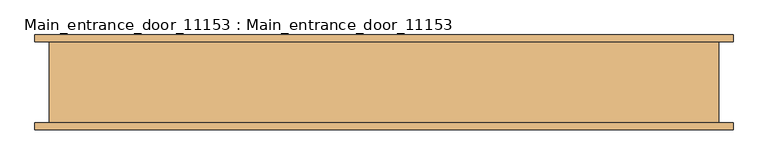
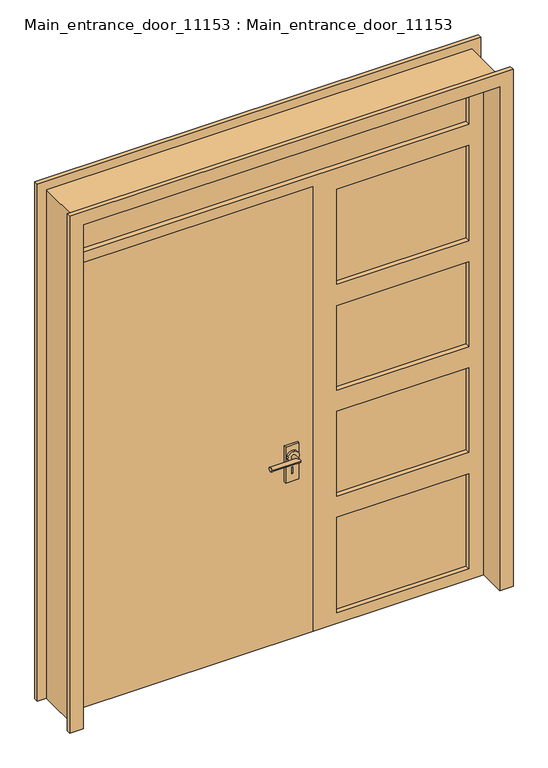
"""IFC4 building model written with IfcOpenShell, lengths in millimetres: door geometry, Main_entrance_door_11153 : Main_entrance_door_11153."""

from ifc_helpers import new_model, si_unit, point, frame, frame_2d, origin, origin_with_axes, place, context, project, spatial, polyline, circle_curve, ellipse_curve, trimmed, segment, composite_curve, outline, extrude, faceted_brep, source, transform, mapped, element, save
from ifc_brep_helpers import plane_surface, cylinder_surface, advanced_brep


def main_entrance_door_11153_main_entrance_door_11153_94c2f9e1(model_context):
    return source(origin(), model_context, "Body", "SolidModel", [
        advanced_brep(
        [(60.0, 60.0, 870.0), (80.0, 60.0, 870.0), (80.0, 100.0, 870.0), (60.0, 80.0, 870.0), (-50.0, 80.0, 870.0), (-50.0, 100.0, 870.0)],
        [
            (0, 1, circle_curve(frame((70.0, 60.0, 870.0), z_axis=(0.0, -1.0, 0.0), x_axis=(1.0, 0.0, 0.0)), 10.0)),
            (1, 0, circle_curve(frame((70.0, 60.0, 870.0), z_axis=(0.0, -1.0, 0.0), x_axis=(1.0, 0.0, 0.0)), 10.0)),
            (1, 2),
            (2, 3, ellipse_curve(frame((70.0, 90.0, 870.0), z_axis=(0.7071067811865411, -0.7071067811865538, 0.0), x_axis=(-0.7071067811865538, -0.7071067811865412, 0.0)), 14.1421356, 10.0)),
            (3, 0),
            (3, 2, ellipse_curve(frame((70.0, 90.0, 870.0), z_axis=(0.7071067811865411, -0.7071067811865538, 0.0), x_axis=(-0.7071067811865538, -0.7071067811865412, 0.0)), 14.1421356, 10.0)),
            (4, 5, circle_curve(frame((-50.0, 90.0, 870.0), z_axis=(-1.0, 0.0, 0.0), x_axis=(0.0, 1.0, 0.0)), 10.0)),
            (5, 4, circle_curve(frame((-50.0, 90.0, 870.0), z_axis=(-1.0, 0.0, 0.0), x_axis=(0.0, 1.0, 0.0)), 10.0)),
            (2, 5),
            (4, 3),
        ],
        [
            plane_surface(frame((70.0, 60.0, 870.0), z_axis=(0.0, -1.0, 0.0), x_axis=(0.0, 0.0, 1.0))),
            cylinder_surface(frame((70.0, 60.0, 870.0), z_axis=(0.0, -1.0, 0.0), x_axis=(1.0, 0.0, 0.0)), 10.0),
            plane_surface(frame((-50.0, 90.0, 870.0), z_axis=(-1.0, 0.0, 0.0), x_axis=(0.0, 0.0, 1.0))),
            cylinder_surface(frame((70.0, 90.0, 870.0), z_axis=(1.0, 0.0, 0.0), x_axis=(0.0, 1.0, 0.0)), 10.0),
        ],
        [
            (0, [[1, 2]]),
            (1, [[3, 4, 5, -2]]),
            (1, [[-5, 6, -3, -1]]),
            (2, [[7, 8]]),
            (3, [[9, -7, 10, -4]]),
            (3, [[-10, -8, -9, -6]]),
        ],
    ),
        extrude(outline(polyline([(920.0, 100.0), (920.0, 40.0), (750.0, 40.0), (750.0, 100.0), (920.0, 100.0)]), holes=[polyline([(815.3510082, 71.5671262), (785.3510082, 71.5671262), (785.3510082, 68.4328738), (815.3510082, 68.4328738), (815.3510082, 71.5671262)])]), frame((0.0, 40.0, 0.0), z_axis=(0.0, 1.0, 0.0), x_axis=(0.0, 0.0, 1.0)), (0.0, 0.0, 1.0), 10.0),
        extrude(outline(composite_curve([segment(trimmed(circle_curve(frame_2d((870.0, 70.0)), 25.0), [point((870.0, 45.0))], [point((870.0, 95.0))], False, "CARTESIAN"), True, "CONTINUOUS"), segment(trimmed(circle_curve(frame_2d((870.0, 70.0)), 25.0), [point((870.0, 95.0))], [point((870.0, 45.0))], False, "CARTESIAN"), True, "CONTINUOUS")], self_intersect=False)), frame((0.0, 40.0, 0.0), z_axis=(0.0, 1.0, 0.0), x_axis=(0.0, 0.0, 1.0)), (0.0, 0.0, 1.0), 20.0),
        advanced_brep(
        [(60.0, -30.0, 870.0), (80.0, -30.0, 870.0), (60.0, -50.0, 870.0), (80.0, -70.0, 870.0), (-50.0, -50.0, 870.0), (-50.0, -70.0, 870.0)],
        [
            (0, 1, circle_curve(frame((70.0, -30.0, 870.0), z_axis=(0.0, 1.0, 0.0), x_axis=(1.0, 0.0, 0.0)), 10.0)),
            (1, 0, circle_curve(frame((70.0, -30.0, 870.0), z_axis=(0.0, 1.0, 0.0), x_axis=(1.0, 0.0, 0.0)), 10.0)),
            (0, 2),
            (2, 3, ellipse_curve(frame((70.0, -60.0, 870.0), z_axis=(0.7071067811865457, 0.7071067811865492, 0.0), x_axis=(-0.7071067811865492, 0.7071067811865458, 0.0)), 14.1421356, 10.0)),
            (3, 1),
            (3, 2, ellipse_curve(frame((70.0, -60.0, 870.0), z_axis=(0.7071067811865457, 0.7071067811865492, 0.0), x_axis=(-0.7071067811865492, 0.7071067811865458, 0.0)), 14.1421356, 10.0)),
            (4, 5, circle_curve(frame((-50.0, -60.0, 870.0), z_axis=(-1.0, 0.0, 0.0), x_axis=(0.0, -1.0, 0.0)), 10.0)),
            (5, 4, circle_curve(frame((-50.0, -60.0, 870.0), z_axis=(-1.0, 0.0, 0.0), x_axis=(0.0, -1.0, 0.0)), 10.0)),
            (2, 4),
            (5, 3),
        ],
        [
            plane_surface(frame((70.0, -30.0, 870.0), z_axis=(0.0, 1.0, 0.0), x_axis=(0.0, 0.0, 1.0))),
            cylinder_surface(frame((70.0, -30.0, 870.0), z_axis=(0.0, 1.0, 0.0), x_axis=(1.0, 0.0, 0.0)), 10.0),
            plane_surface(frame((-50.0, -60.0, 870.0), z_axis=(-1.0, 0.0, 0.0), x_axis=(0.0, 0.0, 1.0))),
            cylinder_surface(frame((70.0, -60.0, 870.0), z_axis=(1.0, 0.0, 0.0), x_axis=(0.0, -1.0, 0.0)), 10.0),
        ],
        [
            (0, [[1, 2]]),
            (1, [[-1, 3, 4, 5]]),
            (1, [[-2, -5, 6, -3]]),
            (2, [[7, 8]]),
            (3, [[-4, 9, -8, 10]]),
            (3, [[-6, -10, -7, -9]]),
        ],
    ),
        extrude(outline(polyline([(920.0, 100.0), (920.0, 40.0), (750.0, 40.0), (750.0, 100.0), (920.0, 100.0)]), holes=[polyline([(815.3510082, 71.5671262), (785.3510082, 71.5671262), (785.3510082, 68.4328738), (815.3510082, 68.4328738), (815.3510082, 71.5671262)])]), frame((0.0, -20.0, 0.0), z_axis=(0.0, 1.0, 0.0), x_axis=(0.0, 0.0, 1.0)), (0.0, 0.0, 1.0), 10.0),
        extrude(outline(composite_curve([segment(trimmed(circle_curve(frame_2d((870.0, 70.0)), 25.0), [point((870.0, 45.0))], [point((870.0, 95.0))], False, "CARTESIAN"), True, "CONTINUOUS"), segment(trimmed(circle_curve(frame_2d((870.0, 70.0)), 25.0), [point((870.0, 95.0))], [point((870.0, 45.0))], False, "CARTESIAN"), True, "CONTINUOUS")], self_intersect=False)), frame((0.0, -30.0, 0.0), z_axis=(0.0, 1.0, 0.0), x_axis=(0.0, 0.0, 1.0)), (0.0, 0.0, 1.0), 20.0),
        faceted_brep([(990.0, 114.3, 0.0), (950.0, 114.3, 0.0), (950.0, -114.3, 0.0), (990.0, -114.3, 0.0), (990.0, -134.3, 0.0), (930.0, -134.3, 0.0), (930.0, 40.0, 0.0), (915.0, 40.0, 0.0), (915.0, 55.0, 0.0), (930.0, 55.0, 0.0), (930.0, 134.3, 0.0), (990.0, 134.3, 0.0), (990.0, 114.3, 2440.0), (-990.0, 114.3, 2440.0), (-990.0, 114.3, 0.0), (-950.0, 114.3, 0.0), (-950.0, 114.3, 2400.0), (950.0, 114.3, 2400.0), (950.0, -114.3, 2400.0), (-950.0, -114.3, 2400.0), (-950.0, -114.3, 0.0), (-990.0, -114.3, 0.0), (-990.0, -114.3, 2440.0), (990.0, -114.3, 2440.0), (990.0, -134.3, 2440.0), (-990.0, -134.3, 2440.0), (-990.0, -134.3, 0.0), (-930.0, -134.3, 0.0), (-930.0, -134.3, 2380.0), (930.0, -134.3, 2380.0), (930.0, 40.0, 2380.0), (-930.0, 40.0, 2380.0), (-930.0, 40.0, 0.0), (-915.0, 40.0, 0.0), (-915.0, 40.0, 2365.0), (915.0, 40.0, 2365.0), (915.0, 55.0, 2365.0), (-915.0, 55.0, 2365.0), (-915.0, 55.0, 0.0), (-930.0, 55.0, 0.0), (-930.0, 55.0, 2380.0), (930.0, 55.0, 2380.0), (930.0, 134.3, 2380.0), (-930.0, 134.3, 2380.0), (-930.0, 134.3, 0.0), (-990.0, 134.3, 0.0), (-990.0, 134.3, 2440.0), (990.0, 134.3, 2440.0)], [[[0, 1, 2, 3, 4, 5, 6, 7, 8, 9, 10, 11]], [[1, 0, 12, 13, 14, 15, 16, 17]], [[2, 1, 17, 18]], [[3, 2, 18, 19, 20, 21, 22, 23]], [[4, 3, 23, 24]], [[5, 4, 24, 25, 26, 27, 28, 29]], [[6, 5, 29, 30]], [[7, 6, 30, 31, 32, 33, 34, 35]], [[8, 7, 35, 36]], [[9, 8, 36, 37, 38, 39, 40, 41]], [[10, 9, 41, 42]], [[11, 10, 42, 43, 44, 45, 46, 47]], [[0, 11, 47, 12]], [[14, 13, 46, 45]], [[15, 14, 45, 44, 39, 38, 33, 32, 27, 26, 21, 20]], [[16, 15, 20, 19]], [[22, 21, 26, 25]], [[28, 27, 32, 31]], [[34, 33, 38, 37]], [[40, 39, 44, 43]], [[13, 12, 47, 46]], [[17, 16, 19, 18]], [[23, 22, 25, 24]], [[29, 28, 31, 30]], [[35, 34, 37, 36]], [[41, 40, 43, 42]]]),
        faceted_brep([(225.0, 40.0, 0.0), (930.0, 40.0, 0.0), (930.0, -10.0, 0.0), (170.0, -10.0, 0.0), (170.0, 40.0, 0.0), (155.0, 40.0, 0.0), (155.0, 55.0, 0.0), (225.0, 55.0, 0.0), (225.0, 40.0, 2100.0), (930.0, 40.0, 2100.0), (865.0, 40.0, 500.0), (275.0, 40.0, 500.0), (275.0, 40.0, 50.0), (865.0, 40.0, 50.0), (865.0, 40.0, 1000.0), (275.0, 40.0, 1000.0), (275.0, 40.0, 600.0), (865.0, 40.0, 600.0), (865.0, 40.0, 1500.0), (275.0, 40.0, 1500.0), (275.0, 40.0, 1100.0), (865.0, 40.0, 1100.0), (865.0, 40.0, 2050.0), (275.0, 40.0, 2050.0), (275.0, 40.0, 1600.0), (865.0, 40.0, 1600.0), (930.0, 55.0, 2100.0), (930.0, 55.0, 2380.0), (930.0, -10.0, 2380.0), (-930.0, -10.0, 2380.0), (-930.0, -10.0, 2100.0), (170.0, -10.0, 2100.0), (275.0, -10.0, 500.0), (865.0, -10.0, 500.0), (865.0, -10.0, 50.0), (275.0, -10.0, 50.0), (275.0, -10.0, 1000.0), (865.0, -10.0, 1000.0), (865.0, -10.0, 600.0), (275.0, -10.0, 600.0), (-880.0, -10.0, 2315.0), (865.0, -10.0, 2315.0), (865.0, -10.0, 2150.0), (-880.0, -10.0, 2150.0), (275.0, -10.0, 1500.0), (865.0, -10.0, 1500.0), (865.0, -10.0, 1100.0), (275.0, -10.0, 1100.0), (275.0, -10.0, 2050.0), (865.0, -10.0, 2050.0), (865.0, -10.0, 1600.0), (275.0, -10.0, 1600.0), (170.0, 40.0, 2100.0), (155.0, 40.0, 2100.0), (155.0, 55.0, 2100.0), (-930.0, 55.0, 2100.0), (-930.0, 55.0, 2380.0), (225.0, 55.0, 2100.0), (865.0, 55.0, 2315.0), (-880.0, 55.0, 2315.0), (-880.0, 55.0, 2150.0), (865.0, 55.0, 2150.0)], [[[0, 1, 2, 3, 4, 5, 6, 7]], [[1, 0, 8, 9], [10, 11, 12, 13], [14, 15, 16, 17], [18, 19, 20, 21], [22, 23, 24, 25]], [[2, 1, 9, 26, 27, 28]], [[3, 2, 28, 29, 30, 31], [32, 33, 34, 35], [36, 37, 38, 39], [40, 41, 42, 43], [44, 45, 46, 47], [48, 49, 50, 51]], [[4, 3, 31, 52]], [[5, 4, 52, 53]], [[6, 5, 53, 54]], [[7, 6, 54, 55, 56, 27, 26, 57], [58, 59, 60, 61]], [[0, 7, 57, 8]], [[10, 33, 32, 11]], [[33, 10, 13, 34]], [[12, 35, 34, 13]], [[11, 32, 35, 12]], [[14, 37, 36, 15]], [[37, 14, 17, 38]], [[16, 39, 38, 17]], [[15, 36, 39, 16]], [[45, 18, 21, 46]], [[20, 47, 46, 21]], [[19, 44, 47, 20]], [[27, 56, 29, 28]], [[29, 56, 55, 30]], [[58, 41, 40, 59]], [[41, 58, 61, 42]], [[59, 40, 43, 60]], [[18, 45, 44, 19]], [[22, 49, 48, 23]], [[24, 51, 50, 25]], [[23, 48, 51, 24]], [[49, 22, 25, 50]], [[57, 26, 9, 8]], [[30, 55, 54, 53, 52, 31]], [[60, 43, 42, 61]]]),
        extrude(outline(polyline([(170.0, 40.0), (170.0, -10.0), (-930.0, -10.0), (-930.0, 40.0), (170.0, 40.0)])), origin_with_axes(), (0.0, 0.0, 1.0), 2100.0),
        extrude(outline(polyline([(-880.0, 12.0), (-880.0, 18.0), (865.0, 18.0), (865.0, 12.0), (-880.0, 12.0)])), frame((0.0, 0.0, 2150.0), z_axis=(0.0, 0.0, 1.0), x_axis=(1.0, 0.0, 0.0)), (0.0, 0.0, 1.0), 165.0),
        extrude(outline(polyline([(865.0, 18.0), (865.0, 12.0), (275.0, 12.0), (275.0, 18.0), (865.0, 18.0)])), frame((0.0, 0.0, 50.0), z_axis=(0.0, 0.0, 1.0), x_axis=(1.0, 0.0, 0.0)), (0.0, 0.0, 1.0), 450.0),
        extrude(outline(polyline([(865.0, 18.0), (865.0, 12.0), (275.0, 12.0), (275.0, 18.0), (865.0, 18.0)])), frame((0.0, 0.0, 600.0), z_axis=(0.0, 0.0, 1.0), x_axis=(1.0, 0.0, 0.0)), (0.0, 0.0, 1.0), 400.0),
        extrude(outline(polyline([(865.0, 18.0), (865.0, 12.0), (275.0, 12.0), (275.0, 18.0), (865.0, 18.0)])), frame((0.0, 0.0, 1600.0), z_axis=(0.0, 0.0, 1.0), x_axis=(1.0, 0.0, 0.0)), (0.0, 0.0, 1.0), 450.0),
        extrude(outline(polyline([(865.0, 18.0), (865.0, 12.0), (275.0, 12.0), (275.0, 18.0), (865.0, 18.0)])), frame((0.0, 0.0, 1100.0), z_axis=(0.0, 0.0, 1.0), x_axis=(1.0, 0.0, 0.0)), (0.0, 0.0, 1.0), 400.0),
    ])


if __name__ == "__main__":
    model = new_model("IFC4")
    model_context = context("Model", 3, world=origin())
    ifc_project = project(units=[si_unit("LENGTHUNIT", "METRE", prefix="MILLI")], contexts=[model_context])
    site = spatial("IfcSite", under=ifc_project)
    building = spatial("IfcBuilding", under=site)
    placement = place(None, origin())
    main_entrance_door_11153_main_entrance_door_11153_shape = main_entrance_door_11153_main_entrance_door_11153_94c2f9e1(model_context)
    element("IfcDoor", 1, ObjectType="Main_entrance_door_11153 : Main_entrance_door_11153", at=placement, inside=building, context=model_context, shape_type="MappedRepresentation", body=[
        mapped(main_entrance_door_11153_main_entrance_door_11153_shape, transform((0.0, 0.0, 0.0), x_axis=(1.0, 0.0, 0.0), y_axis=(0.0, 1.0, 0.0), z_axis=(0.0, 0.0, 1.0))),
    ])
    save(model, "model.ifc")

# Revit data of these elements
# Type "Main_entrance_door_11153 : Main_entrance_door_11153"
#   Type Mark = "14"
#   Height = 7' - 10.48819"
#   Width = 6' - 2.80315"
#   Door Width = 3' - 7.30709"
#   Function = (empty or 0)
#   Wall Closure = (empty or 0)
# Element 1 (IfcDoor, "Main_entrance_door_11153 : Main_entrance_door_11153")
#   Materials on its faces: "Glass", "Default"
# Materials
#   "Glass": class "Glass", colour RGB 0 128 192, transparency 0.75, Description = "Soda Lime Glass", Cost = 0
#   "Default": colour RGB 127 127 127, transparency 0, Cost = 0
